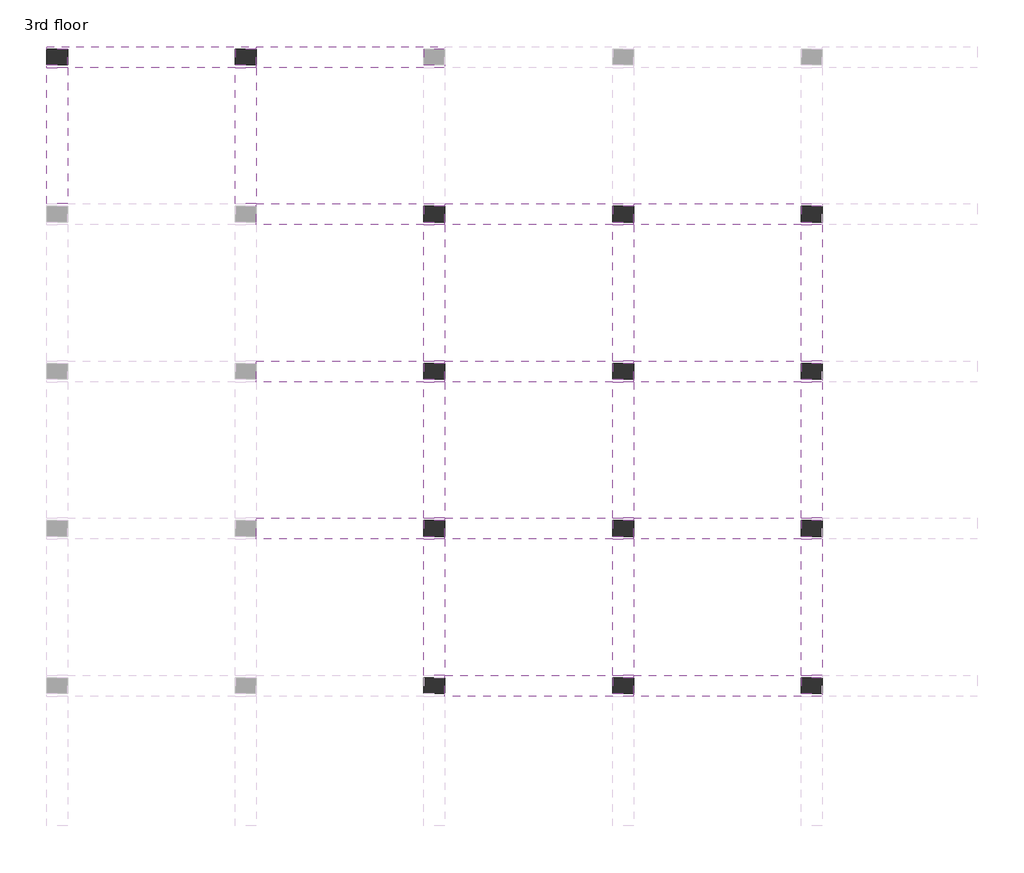
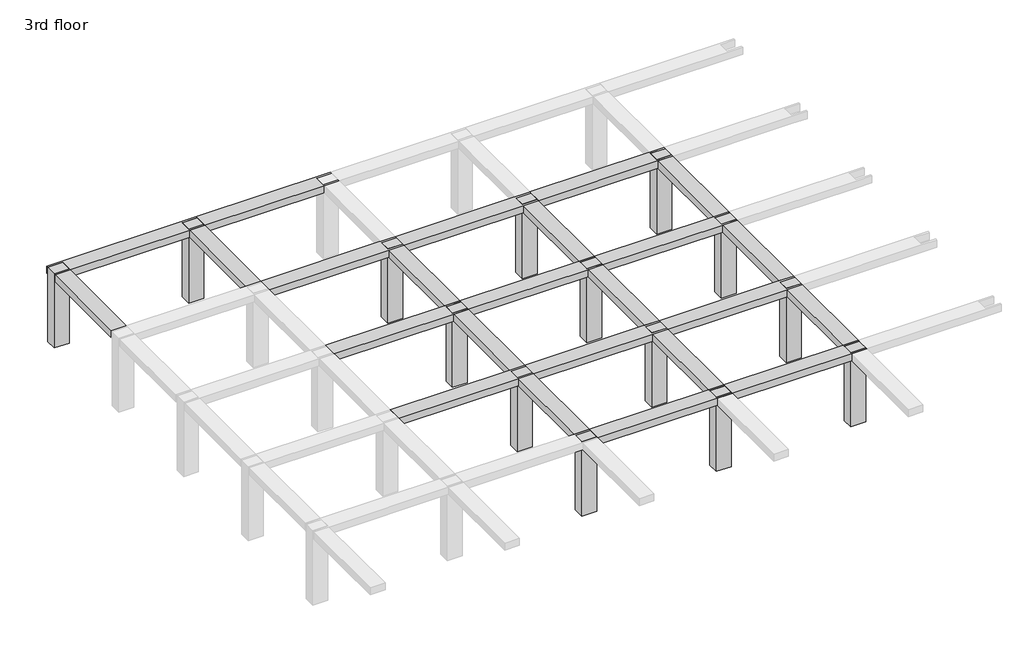
# One storey, part 2 of 3: 24 beams, 14 columns.
"""IFC4 building model written with IfcOpenShell, lengths in millimetres."""

from ifc_helpers import new_model, si_unit, frame, origin, place, context, project, spatial, polyline, outline, extrude, faceted_brep, element, save

model = new_model("IFC4")

# Units and contexts
model_context = context("Model", 3, world=origin())
ifc_project = project(units=[si_unit("LENGTHUNIT", "METRE", prefix="MILLI")], contexts=[model_context])

# Site, building, storey
site = spatial("IfcSite", under=ifc_project)
building = spatial("IfcBuilding", under=site)
storey = spatial("IfcBuildingStorey", under=building, Name="3rd floor", Elevation=9601.2)

# Beams
placement = place(None, origin())
element("IfcBeam", 1, ObjectType="Concrete-Rectangular Beam : 2' x2'", at=placement, inside=storey, context=model_context, shape_type="Brep", body=[
    faceted_brep([(-5646.474232, 1680.7831222, 12801.6), (-6256.074232, 1680.7831222, 12801.6), (-11132.874232, 1680.7831222, 12801.6), (-11132.874232, 1604.5831222, 12801.6), (-11132.874232, 1147.3831222, 12801.6), (-11132.874232, 1071.1831222, 12801.6), (-6256.074232, 1071.1831222, 12801.6), (-5646.474232, 1071.1831222, 12801.6), (-5646.474232, 1147.3831222, 12801.6), (-6256.074232, 1147.3831222, 12801.6), (-6256.074232, 1604.5831222, 12801.6), (-5646.474232, 1604.5831222, 12801.6), (-5646.474232, 1071.1831222, 12496.8), (-11132.874232, 1071.1831222, 12496.8), (-6256.074232, 1071.1831222, 12496.8), (-11132.874232, 1147.3831222, 12496.8), (-11132.874232, 1604.5831222, 12496.8), (-11132.874232, 1680.7831222, 12496.8), (-6256.074232, 1680.7831222, 12496.8), (-5646.474232, 1680.7831222, 12496.8), (-5646.474232, 1604.5831222, 12496.8), (-6256.074232, 1604.5831222, 12496.8), (-6256.074232, 1147.3831222, 12496.8), (-5646.474232, 1147.3831222, 12496.8)], [[[0, 1, 2, 3, 4, 5, 6, 7, 8, 9, 10, 11]], [[12, 7, 6, 5, 13, 14]], [[12, 14, 13, 15, 16, 17, 18, 19, 20, 21, 22, 23]], [[0, 19, 18, 17, 2, 1]], [[7, 12, 23, 8]], [[5, 4, 3, 2, 17, 16, 15, 13]], [[22, 9, 8, 23]], [[9, 22, 21, 10]], [[10, 21, 20, 11]], [[19, 0, 11, 20]]]),
])
element("IfcBeam", 2, ObjectType="Concrete-Rectangular Beam : 2' x2'", at=placement, inside=storey, context=model_context, shape_type="Brep", body=[
    faceted_brep([(-5646.474232, 1680.7831222, 12801.6), (-5646.474232, 1604.5831222, 12801.6), (-5646.474232, 1147.3831222, 12801.6), (-5646.474232, 1071.1831222, 12801.6), (-769.674232, 1071.1831222, 12801.6), (-160.074232, 1071.1831222, 12801.6), (-160.074232, 1147.3831222, 12801.6), (-769.674232, 1147.3831222, 12801.6), (-769.674232, 1604.5831222, 12801.6), (-160.074232, 1604.5831222, 12801.6), (-160.074232, 1680.7831222, 12801.6), (-769.674232, 1680.7831222, 12801.6), (-5646.474232, 1071.1831222, 12496.8), (-769.674232, 1071.1831222, 12496.8), (-160.074232, 1071.1831222, 12496.8), (-5646.474232, 1147.3831222, 12496.8), (-5646.474232, 1604.5831222, 12496.8), (-5646.474232, 1680.7831222, 12496.8), (-769.674232, 1680.7831222, 12496.8), (-160.074232, 1680.7831222, 12496.8), (-160.074232, 1604.5831222, 12496.8), (-769.674232, 1604.5831222, 12496.8), (-769.674232, 1147.3831222, 12496.8), (-160.074232, 1147.3831222, 12496.8)], [[[0, 1, 2, 3, 4, 5, 6, 7, 8, 9, 10, 11]], [[3, 12, 13, 14, 5, 4]], [[12, 15, 16, 17, 18, 19, 20, 21, 22, 23, 14, 13]], [[10, 19, 18, 17, 0, 11]], [[3, 2, 1, 0, 17, 16, 15, 12]], [[5, 14, 23, 6]], [[22, 7, 6, 23]], [[7, 22, 21, 8]], [[8, 21, 20, 9]], [[19, 10, 9, 20]]]),
])
element("IfcBeam", 3, ObjectType="Concrete-Rectangular Beam : 2' x2'", at=placement, inside=storey, context=model_context, shape_type="Brep", body=[
    faceted_brep([(-16619.274232, 6252.7831222, 12801.6), (-16619.274232, 6176.5831222, 12801.6), (-16619.274232, 5719.3831222, 12801.6), (-16619.274232, 5643.1831222, 12801.6), (-11742.474232, 5643.1831222, 12801.6), (-11132.874232, 5643.1831222, 12801.6), (-11132.874232, 5719.3831222, 12801.6), (-11742.474232, 5719.3831222, 12801.6), (-11742.474232, 6176.5831222, 12801.6), (-11132.874232, 6176.5831222, 12801.6), (-11132.874232, 6252.7831222, 12801.6), (-11742.474232, 6252.7831222, 12801.6), (-16619.274232, 5643.1831222, 12496.8), (-11742.474232, 5643.1831222, 12496.8), (-11132.874232, 5643.1831222, 12496.8), (-16619.274232, 5719.3831222, 12496.8), (-16619.274232, 6176.5831222, 12496.8), (-16619.274232, 6252.7831222, 12496.8), (-11742.474232, 6252.7831222, 12496.8), (-11132.874232, 6252.7831222, 12496.8), (-11132.874232, 6176.5831222, 12496.8), (-11742.474232, 6176.5831222, 12496.8), (-11742.474232, 5719.3831222, 12496.8), (-11132.874232, 5719.3831222, 12496.8)], [[[0, 1, 2, 3, 4, 5, 6, 7, 8, 9, 10, 11]], [[3, 12, 13, 14, 5, 4]], [[12, 15, 16, 17, 18, 19, 20, 21, 22, 23, 14, 13]], [[10, 19, 18, 17, 0, 11]], [[3, 2, 1, 0, 17, 16, 15, 12]], [[5, 14, 23, 6]], [[22, 7, 6, 23]], [[7, 22, 21, 8]], [[8, 21, 20, 9]], [[19, 10, 9, 20]]]),
])
element("IfcBeam", 4, ObjectType="Concrete-Rectangular Beam : 2' x2'", at=placement, inside=storey, context=model_context, shape_type="Brep", body=[
    faceted_brep([(-5646.474232, 6252.7831222, 12801.6), (-6256.074232, 6252.7831222, 12801.6), (-11132.874232, 6252.7831222, 12801.6), (-11132.874232, 6176.5831222, 12801.6), (-11132.874232, 5719.3831222, 12801.6), (-11132.874232, 5643.1831222, 12801.6), (-6256.074232, 5643.1831222, 12801.6), (-5646.474232, 5643.1831222, 12801.6), (-5646.474232, 5719.3831222, 12801.6), (-6256.074232, 5719.3831222, 12801.6), (-6256.074232, 6176.5831222, 12801.6), (-5646.474232, 6176.5831222, 12801.6), (-5646.474232, 5643.1831222, 12496.8), (-11132.874232, 5643.1831222, 12496.8), (-6256.074232, 5643.1831222, 12496.8), (-11132.874232, 5719.3831222, 12496.8), (-11132.874232, 6176.5831222, 12496.8), (-11132.874232, 6252.7831222, 12496.8), (-6256.074232, 6252.7831222, 12496.8), (-5646.474232, 6252.7831222, 12496.8), (-5646.474232, 6176.5831222, 12496.8), (-6256.074232, 6176.5831222, 12496.8), (-6256.074232, 5719.3831222, 12496.8), (-5646.474232, 5719.3831222, 12496.8)], [[[0, 1, 2, 3, 4, 5, 6, 7, 8, 9, 10, 11]], [[12, 7, 6, 5, 13, 14]], [[12, 14, 13, 15, 16, 17, 18, 19, 20, 21, 22, 23]], [[0, 19, 18, 17, 2, 1]], [[7, 12, 23, 8]], [[5, 4, 3, 2, 17, 16, 15, 13]], [[22, 9, 8, 23]], [[9, 22, 21, 10]], [[10, 21, 20, 11]], [[19, 0, 11, 20]]]),
])
element("IfcBeam", 5, ObjectType="Concrete-Rectangular Beam : 2' x2'", at=placement, inside=storey, context=model_context, shape_type="Brep", body=[
    faceted_brep([(-5646.474232, 6252.7831222, 12801.6), (-5646.474232, 6176.5831222, 12801.6), (-5646.474232, 5719.3831222, 12801.6), (-5646.474232, 5643.1831222, 12801.6), (-769.674232, 5643.1831222, 12801.6), (-160.074232, 5643.1831222, 12801.6), (-160.074232, 5719.3831222, 12801.6), (-769.674232, 5719.3831222, 12801.6), (-769.674232, 6176.5831222, 12801.6), (-160.074232, 6176.5831222, 12801.6), (-160.074232, 6252.7831222, 12801.6), (-769.674232, 6252.7831222, 12801.6), (-5646.474232, 5643.1831222, 12496.8), (-769.674232, 5643.1831222, 12496.8), (-160.074232, 5643.1831222, 12496.8), (-5646.474232, 5719.3831222, 12496.8), (-5646.474232, 6176.5831222, 12496.8), (-5646.474232, 6252.7831222, 12496.8), (-769.674232, 6252.7831222, 12496.8), (-160.074232, 6252.7831222, 12496.8), (-160.074232, 6176.5831222, 12496.8), (-769.674232, 6176.5831222, 12496.8), (-769.674232, 5719.3831222, 12496.8), (-160.074232, 5719.3831222, 12496.8)], [[[0, 1, 2, 3, 4, 5, 6, 7, 8, 9, 10, 11]], [[3, 12, 13, 14, 5, 4]], [[12, 15, 16, 17, 18, 19, 20, 21, 22, 23, 14, 13]], [[10, 19, 18, 17, 0, 11]], [[3, 2, 1, 0, 17, 16, 15, 12]], [[5, 14, 23, 6]], [[22, 7, 6, 23]], [[7, 22, 21, 8]], [[8, 21, 20, 9]], [[19, 10, 9, 20]]]),
])
element("IfcBeam", 6, ObjectType="Concrete-Rectangular Beam : 2' x2'", at=placement, inside=storey, context=model_context, shape_type="Brep", body=[
    faceted_brep([(-16619.274232, 10824.7831222, 12801.6), (-16619.274232, 10748.5831222, 12801.6), (-16619.274232, 10291.3831222, 12801.6), (-16619.274232, 10215.1831222, 12801.6), (-11742.474232, 10215.1831222, 12801.6), (-11132.874232, 10215.1831222, 12801.6), (-11132.874232, 10291.3831222, 12801.6), (-11742.474232, 10291.3831222, 12801.6), (-11742.474232, 10748.5831222, 12801.6), (-11132.874232, 10748.5831222, 12801.6), (-11132.874232, 10824.7831222, 12801.6), (-11742.474232, 10824.7831222, 12801.6), (-16619.274232, 10215.1831222, 12496.8), (-11742.474232, 10215.1831222, 12496.8), (-11132.874232, 10215.1831222, 12496.8), (-16619.274232, 10291.3831222, 12496.8), (-16619.274232, 10748.5831222, 12496.8), (-16619.274232, 10824.7831222, 12496.8), (-11742.474232, 10824.7831222, 12496.8), (-11132.874232, 10824.7831222, 12496.8), (-11132.874232, 10748.5831222, 12496.8), (-11742.474232, 10748.5831222, 12496.8), (-11742.474232, 10291.3831222, 12496.8), (-11132.874232, 10291.3831222, 12496.8)], [[[0, 1, 2, 3, 4, 5, 6, 7, 8, 9, 10, 11]], [[3, 12, 13, 14, 5, 4]], [[12, 15, 16, 17, 18, 19, 20, 21, 22, 23, 14, 13]], [[10, 19, 18, 17, 0, 11]], [[3, 2, 1, 0, 17, 16, 15, 12]], [[5, 14, 23, 6]], [[22, 7, 6, 23]], [[7, 22, 21, 8]], [[8, 21, 20, 9]], [[19, 10, 9, 20]]]),
])
element("IfcBeam", 7, ObjectType="Concrete-Rectangular Beam : 2' x2'", at=placement, inside=storey, context=model_context, shape_type="Brep", body=[
    faceted_brep([(-11132.874232, 10824.7831222, 12801.6), (-11132.874232, 10748.5831222, 12801.6), (-11132.874232, 10291.3831222, 12801.6), (-11132.874232, 10215.1831222, 12801.6), (-6256.074232, 10215.1831222, 12801.6), (-5646.474232, 10215.1831222, 12801.6), (-5646.474232, 10291.3831222, 12801.6), (-6256.074232, 10291.3831222, 12801.6), (-6256.074232, 10748.5831222, 12801.6), (-5646.474232, 10748.5831222, 12801.6), (-5646.474232, 10824.7831222, 12801.6), (-6256.074232, 10824.7831222, 12801.6), (-11132.874232, 10215.1831222, 12496.8), (-6256.074232, 10215.1831222, 12496.8), (-5646.474232, 10215.1831222, 12496.8), (-11132.874232, 10291.3831222, 12496.8), (-11132.874232, 10748.5831222, 12496.8), (-11132.874232, 10824.7831222, 12496.8), (-6256.074232, 10824.7831222, 12496.8), (-5646.474232, 10824.7831222, 12496.8), (-5646.474232, 10748.5831222, 12496.8), (-6256.074232, 10748.5831222, 12496.8), (-6256.074232, 10291.3831222, 12496.8), (-5646.474232, 10291.3831222, 12496.8)], [[[0, 1, 2, 3, 4, 5, 6, 7, 8, 9, 10, 11]], [[3, 12, 13, 14, 5, 4]], [[12, 15, 16, 17, 18, 19, 20, 21, 22, 23, 14, 13]], [[10, 19, 18, 17, 0, 11]], [[3, 2, 1, 0, 17, 16, 15, 12]], [[5, 14, 23, 6]], [[22, 7, 6, 23]], [[7, 22, 21, 8]], [[8, 21, 20, 9]], [[19, 10, 9, 20]]]),
])
element("IfcBeam", 8, ObjectType="Concrete-Rectangular Beam : 2' x2'", at=placement, inside=storey, context=model_context, shape_type="Brep", body=[
    faceted_brep([(-5646.474232, 10824.7831222, 12801.6), (-5646.474232, 10748.5831222, 12801.6), (-5646.474232, 10291.3831222, 12801.6), (-5646.474232, 10215.1831222, 12801.6), (-769.674232, 10215.1831222, 12801.6), (-160.074232, 10215.1831222, 12801.6), (-160.074232, 10291.3831222, 12801.6), (-769.674232, 10291.3831222, 12801.6), (-769.674232, 10748.5831222, 12801.6), (-160.074232, 10748.5831222, 12801.6), (-160.074232, 10824.7831222, 12801.6), (-769.674232, 10824.7831222, 12801.6), (-5646.474232, 10215.1831222, 12496.8), (-769.674232, 10215.1831222, 12496.8), (-160.074232, 10215.1831222, 12496.8), (-5646.474232, 10291.3831222, 12496.8), (-5646.474232, 10748.5831222, 12496.8), (-5646.474232, 10824.7831222, 12496.8), (-769.674232, 10824.7831222, 12496.8), (-160.074232, 10824.7831222, 12496.8), (-160.074232, 10748.5831222, 12496.8), (-769.674232, 10748.5831222, 12496.8), (-769.674232, 10291.3831222, 12496.8), (-160.074232, 10291.3831222, 12496.8)], [[[0, 1, 2, 3, 4, 5, 6, 7, 8, 9, 10, 11]], [[3, 12, 13, 14, 5, 4]], [[12, 15, 16, 17, 18, 19, 20, 21, 22, 23, 14, 13]], [[10, 19, 18, 17, 0, 11]], [[3, 2, 1, 0, 17, 16, 15, 12]], [[5, 14, 23, 6]], [[22, 7, 6, 23]], [[7, 22, 21, 8]], [[8, 21, 20, 9]], [[19, 10, 9, 20]]]),
])
element("IfcBeam", 9, ObjectType="Concrete-Rectangular Beam : 2' x2'", at=placement, inside=storey, context=model_context, shape_type="Brep", body=[
    faceted_brep([(-16619.274232, 15396.7831222, 12801.6), (-16619.274232, 15320.5831222, 12801.6), (-16619.274232, 14863.3831222, 12801.6), (-16619.274232, 14787.1831222, 12801.6), (-11742.474232, 14787.1831222, 12801.6), (-11132.874232, 14787.1831222, 12801.6), (-11132.874232, 14863.3831222, 12801.6), (-11742.474232, 14863.3831222, 12801.6), (-11742.474232, 15320.5831222, 12801.6), (-11132.874232, 15320.5831222, 12801.6), (-11132.874232, 15396.7831222, 12801.6), (-11742.474232, 15396.7831222, 12801.6), (-16619.274232, 14787.1831222, 12496.8), (-11742.474232, 14787.1831222, 12496.8), (-11132.874232, 14787.1831222, 12496.8), (-16619.274232, 14863.3831222, 12496.8), (-16619.274232, 15320.5831222, 12496.8), (-16619.274232, 15396.7831222, 12496.8), (-11742.474232, 15396.7831222, 12496.8), (-11132.874232, 15396.7831222, 12496.8), (-11132.874232, 15320.5831222, 12496.8), (-11742.474232, 15320.5831222, 12496.8), (-11742.474232, 14863.3831222, 12496.8), (-11132.874232, 14863.3831222, 12496.8)], [[[0, 1, 2, 3, 4, 5, 6, 7, 8, 9, 10, 11]], [[3, 12, 13, 14, 5, 4]], [[12, 15, 16, 17, 18, 19, 20, 21, 22, 23, 14, 13]], [[10, 19, 18, 17, 0, 11]], [[3, 2, 1, 0, 17, 16, 15, 12]], [[5, 14, 23, 6]], [[22, 7, 6, 23]], [[7, 22, 21, 8]], [[8, 21, 20, 9]], [[19, 10, 9, 20]]]),
])
element("IfcBeam", 10, ObjectType="Concrete-Rectangular Beam : 2' x2'", at=placement, inside=storey, context=model_context, shape_type="Brep", body=[
    faceted_brep([(-11132.874232, 15396.7831222, 12801.6), (-11132.874232, 15320.5831222, 12801.6), (-11132.874232, 14863.3831222, 12801.6), (-11132.874232, 14787.1831222, 12801.6), (-6256.074232, 14787.1831222, 12801.6), (-5646.474232, 14787.1831222, 12801.6), (-5646.474232, 14863.3831222, 12801.6), (-6256.074232, 14863.3831222, 12801.6), (-6256.074232, 15320.5831222, 12801.6), (-5646.474232, 15320.5831222, 12801.6), (-5646.474232, 15396.7831222, 12801.6), (-6256.074232, 15396.7831222, 12801.6), (-11132.874232, 14787.1831222, 12496.8), (-6256.074232, 14787.1831222, 12496.8), (-5646.474232, 14787.1831222, 12496.8), (-11132.874232, 14863.3831222, 12496.8), (-11132.874232, 15320.5831222, 12496.8), (-11132.874232, 15396.7831222, 12496.8), (-6256.074232, 15396.7831222, 12496.8), (-5646.474232, 15396.7831222, 12496.8), (-5646.474232, 15320.5831222, 12496.8), (-6256.074232, 15320.5831222, 12496.8), (-6256.074232, 14863.3831222, 12496.8), (-5646.474232, 14863.3831222, 12496.8)], [[[0, 1, 2, 3, 4, 5, 6, 7, 8, 9, 10, 11]], [[3, 12, 13, 14, 5, 4]], [[12, 15, 16, 17, 18, 19, 20, 21, 22, 23, 14, 13]], [[10, 19, 18, 17, 0, 11]], [[3, 2, 1, 0, 17, 16, 15, 12]], [[5, 14, 23, 6]], [[22, 7, 6, 23]], [[7, 22, 21, 8]], [[8, 21, 20, 9]], [[19, 10, 9, 20]]]),
])
element("IfcBeam", 11, ObjectType="Concrete-Rectangular Beam : 2' x2'", at=placement, inside=storey, context=model_context, shape_type="Brep", body=[
    faceted_brep([(-5646.474232, 15396.7831222, 12801.6), (-5646.474232, 15320.5831222, 12801.6), (-5646.474232, 14863.3831222, 12801.6), (-5646.474232, 14787.1831222, 12801.6), (-769.674232, 14787.1831222, 12801.6), (-160.074232, 14787.1831222, 12801.6), (-160.074232, 14863.3831222, 12801.6), (-769.674232, 14863.3831222, 12801.6), (-769.674232, 15320.5831222, 12801.6), (-160.074232, 15320.5831222, 12801.6), (-160.074232, 15396.7831222, 12801.6), (-769.674232, 15396.7831222, 12801.6), (-5646.474232, 14787.1831222, 12496.8), (-769.674232, 14787.1831222, 12496.8), (-160.074232, 14787.1831222, 12496.8), (-5646.474232, 14863.3831222, 12496.8), (-5646.474232, 15320.5831222, 12496.8), (-5646.474232, 15396.7831222, 12496.8), (-769.674232, 15396.7831222, 12496.8), (-160.074232, 15396.7831222, 12496.8), (-160.074232, 15320.5831222, 12496.8), (-769.674232, 15320.5831222, 12496.8), (-769.674232, 14863.3831222, 12496.8), (-160.074232, 14863.3831222, 12496.8)], [[[0, 1, 2, 3, 4, 5, 6, 7, 8, 9, 10, 11]], [[3, 12, 13, 14, 5, 4]], [[12, 15, 16, 17, 18, 19, 20, 21, 22, 23, 14, 13]], [[10, 19, 18, 17, 0, 11]], [[3, 2, 1, 0, 17, 16, 15, 12]], [[5, 14, 23, 6]], [[22, 7, 6, 23]], [[7, 22, 21, 8]], [[8, 21, 20, 9]], [[19, 10, 9, 20]]]),
])
element("IfcBeam", 12, ObjectType="Concrete-Rectangular Beam : 2' x2'", at=placement, inside=storey, context=model_context, shape_type="Brep", body=[
    faceted_brep([(-16619.274232, 19968.7831222, 12801.6), (-22715.274232, 19968.7831222, 12801.6), (-22715.274232, 19892.5831222, 12801.6), (-22105.674232, 19892.5831222, 12801.6), (-22105.674232, 19435.3831222, 12801.6), (-22715.274232, 19435.3831222, 12801.6), (-22715.274232, 19359.1831222, 12801.6), (-22105.674232, 19359.1831222, 12801.6), (-17228.874232, 19359.1831222, 12801.6), (-16619.274232, 19359.1831222, 12801.6), (-16619.274232, 19435.3831222, 12801.6), (-17228.874232, 19435.3831222, 12801.6), (-17228.874232, 19892.5831222, 12801.6), (-16619.274232, 19892.5831222, 12801.6), (-22715.274232, 19359.1831222, 12496.8), (-22105.674232, 19359.1831222, 12496.8), (-17228.874232, 19359.1831222, 12496.8), (-16619.274232, 19359.1831222, 12496.8), (-22715.274232, 19435.3831222, 12496.8), (-22105.674232, 19435.3831222, 12496.8), (-22105.674232, 19892.5831222, 12496.8), (-22715.274232, 19892.5831222, 12496.8), (-22715.274232, 19968.7831222, 12496.8), (-16619.274232, 19968.7831222, 12496.8), (-16619.274232, 19892.5831222, 12496.8), (-17228.874232, 19892.5831222, 12496.8), (-17228.874232, 19435.3831222, 12496.8), (-16619.274232, 19435.3831222, 12496.8)], [[[0, 1, 2, 3, 4, 5, 6, 7, 8, 9, 10, 11, 12, 13]], [[6, 14, 15, 16, 17, 9, 8, 7]], [[17, 16, 15, 14, 18, 19, 20, 21, 22, 23, 24, 25, 26, 27]], [[22, 1, 0, 23]], [[14, 6, 5, 18]], [[9, 17, 27, 10]], [[19, 4, 3, 20]], [[4, 19, 18, 5]], [[20, 3, 2, 21]], [[1, 22, 21, 2]], [[26, 11, 10, 27]], [[11, 26, 25, 12]], [[12, 25, 24, 13]], [[23, 0, 13, 24]]]),
])
element("IfcBeam", 13, ObjectType="Concrete-Rectangular Beam : 2' x2'", at=placement, inside=storey, context=model_context, shape_type="Brep", body=[
    faceted_brep([(-11132.874232, 19968.7831222, 12801.6), (-16619.274232, 19968.7831222, 12801.6), (-16619.274232, 19892.5831222, 12801.6), (-16619.274232, 19435.3831222, 12801.6), (-16619.274232, 19359.1831222, 12801.6), (-11742.474232, 19359.1831222, 12801.6), (-11132.874232, 19359.1831222, 12801.6), (-11132.874232, 19435.3831222, 12801.6), (-11742.474232, 19435.3831222, 12801.6), (-11742.474232, 19892.5831222, 12801.6), (-11132.874232, 19892.5831222, 12801.6), (-11132.874232, 19359.1831222, 12496.8), (-16619.274232, 19359.1831222, 12496.8), (-11742.474232, 19359.1831222, 12496.8), (-16619.274232, 19435.3831222, 12496.8), (-16619.274232, 19892.5831222, 12496.8), (-16619.274232, 19968.7831222, 12496.8), (-11132.874232, 19968.7831222, 12496.8), (-11132.874232, 19892.5831222, 12496.8), (-11742.474232, 19892.5831222, 12496.8), (-11742.474232, 19435.3831222, 12496.8), (-11132.874232, 19435.3831222, 12496.8)], [[[0, 1, 2, 3, 4, 5, 6, 7, 8, 9, 10]], [[11, 6, 5, 4, 12, 13]], [[11, 13, 12, 14, 15, 16, 17, 18, 19, 20, 21]], [[0, 17, 16, 1]], [[6, 11, 21, 7]], [[4, 3, 2, 1, 16, 15, 14, 12]], [[20, 8, 7, 21]], [[8, 20, 19, 9]], [[9, 19, 18, 10]], [[17, 0, 10, 18]]]),
])
element("IfcBeam", 14, ObjectType="Concrete-Rectangular Beam : 2' x2'", at=placement, inside=storey, context=model_context, shape_type="SweptSolid", body=[
    extrude(outline(polyline([(-22105.674232, 15396.7831222), (-22715.274232, 15396.7831222), (-22715.274232, 19359.1831222), (-22105.674232, 19359.1831222), (-22105.674232, 15396.7831222)])), frame((0.0, 0.0, 12496.8), z_axis=(0.0, 0.0, 1.0), x_axis=(1.0, 0.0, 0.0)), (0.0, 0.0, 1.0), 304.8),
])
element("IfcBeam", 15, ObjectType="Concrete-Rectangular Beam : 2' x2'", at=placement, inside=storey, context=model_context, shape_type="SweptSolid", body=[
    extrude(outline(polyline([(-16619.274232, 15396.7831222), (-17228.874232, 15396.7831222), (-17228.874232, 19359.1831222), (-16619.274232, 19359.1831222), (-16619.274232, 15396.7831222)])), frame((0.0, 0.0, 12496.8), z_axis=(0.0, 0.0, 1.0), x_axis=(1.0, 0.0, 0.0)), (0.0, 0.0, 1.0), 304.8),
])
element("IfcBeam", 16, ObjectType="Concrete-Rectangular Beam : 2' x2'", at=placement, inside=storey, context=model_context, shape_type="SweptSolid", body=[
    extrude(outline(polyline([(-11132.874232, 1680.7831222), (-11742.474232, 1680.7831222), (-11742.474232, 5643.1831222), (-11132.874232, 5643.1831222), (-11132.874232, 1680.7831222)])), frame((0.0, 0.0, 12496.8), z_axis=(0.0, 0.0, 1.0), x_axis=(1.0, 0.0, 0.0)), (0.0, 0.0, 1.0), 304.8),
])
element("IfcBeam", 17, ObjectType="Concrete-Rectangular Beam : 2' x2'", at=placement, inside=storey, context=model_context, shape_type="SweptSolid", body=[
    extrude(outline(polyline([(-11132.874232, 6252.7831222), (-11742.474232, 6252.7831222), (-11742.474232, 10215.1831222), (-11132.874232, 10215.1831222), (-11132.874232, 6252.7831222)])), frame((0.0, 0.0, 12496.8), z_axis=(0.0, 0.0, 1.0), x_axis=(1.0, 0.0, 0.0)), (0.0, 0.0, 1.0), 304.8),
])
element("IfcBeam", 18, ObjectType="Concrete-Rectangular Beam : 2' x2'", at=placement, inside=storey, context=model_context, shape_type="SweptSolid", body=[
    extrude(outline(polyline([(-11132.874232, 10824.7831222), (-11742.474232, 10824.7831222), (-11742.474232, 14787.1831222), (-11132.874232, 14787.1831222), (-11132.874232, 10824.7831222)])), frame((0.0, 0.0, 12496.8), z_axis=(0.0, 0.0, 1.0), x_axis=(1.0, 0.0, 0.0)), (0.0, 0.0, 1.0), 304.8),
])
element("IfcBeam", 19, ObjectType="Concrete-Rectangular Beam : 2' x2'", at=placement, inside=storey, context=model_context, shape_type="SweptSolid", body=[
    extrude(outline(polyline([(-5646.474232, 1680.7831222), (-6256.074232, 1680.7831222), (-6256.074232, 5643.1831222), (-5646.474232, 5643.1831222), (-5646.474232, 1680.7831222)])), frame((0.0, 0.0, 12496.8), z_axis=(0.0, 0.0, 1.0), x_axis=(1.0, 0.0, 0.0)), (0.0, 0.0, 1.0), 304.8),
])
element("IfcBeam", 20, ObjectType="Concrete-Rectangular Beam : 2' x2'", at=placement, inside=storey, context=model_context, shape_type="SweptSolid", body=[
    extrude(outline(polyline([(-5646.474232, 6252.7831222), (-6256.074232, 6252.7831222), (-6256.074232, 10215.1831222), (-5646.474232, 10215.1831222), (-5646.474232, 6252.7831222)])), frame((0.0, 0.0, 12496.8), z_axis=(0.0, 0.0, 1.0), x_axis=(1.0, 0.0, 0.0)), (0.0, 0.0, 1.0), 304.8),
])
element("IfcBeam", 21, ObjectType="Concrete-Rectangular Beam : 2' x2'", at=placement, inside=storey, context=model_context, shape_type="SweptSolid", body=[
    extrude(outline(polyline([(-5646.474232, 10824.7831222), (-6256.074232, 10824.7831222), (-6256.074232, 14787.1831222), (-5646.474232, 14787.1831222), (-5646.474232, 10824.7831222)])), frame((0.0, 0.0, 12496.8), z_axis=(0.0, 0.0, 1.0), x_axis=(1.0, 0.0, 0.0)), (0.0, 0.0, 1.0), 304.8),
])
element("IfcBeam", 22, ObjectType="Concrete-Rectangular Beam : 2' x2'", at=placement, inside=storey, context=model_context, shape_type="SweptSolid", body=[
    extrude(outline(polyline([(-769.674232, 5643.1831222), (-160.074232, 5643.1831222), (-160.074232, 1680.7831222), (-769.674232, 1680.7831222), (-769.674232, 5643.1831222)])), frame((0.0, 0.0, 12496.8), z_axis=(0.0, 0.0, 1.0), x_axis=(1.0, 0.0, 0.0)), (0.0, 0.0, 1.0), 304.8),
])
element("IfcBeam", 23, ObjectType="Concrete-Rectangular Beam : 2' x2'", at=placement, inside=storey, context=model_context, shape_type="SweptSolid", body=[
    extrude(outline(polyline([(-160.074232, 6252.7831222), (-769.674232, 6252.7831222), (-769.674232, 10215.1831222), (-160.074232, 10215.1831222), (-160.074232, 6252.7831222)])), frame((0.0, 0.0, 12496.8), z_axis=(0.0, 0.0, 1.0), x_axis=(1.0, 0.0, 0.0)), (0.0, 0.0, 1.0), 304.8),
])
element("IfcBeam", 24, ObjectType="Concrete-Rectangular Beam : 2' x2'", at=placement, inside=storey, context=model_context, shape_type="SweptSolid", body=[
    extrude(outline(polyline([(-769.674232, 14787.1831222), (-160.074232, 14787.1831222), (-160.074232, 10824.7831222), (-769.674232, 10824.7831222), (-769.674232, 14787.1831222)])), frame((0.0, 0.0, 12496.8), z_axis=(0.0, 0.0, 1.0), x_axis=(1.0, 0.0, 0.0)), (0.0, 0.0, 1.0), 304.8),
])

# Columns
element("IfcColumn", 25, ObjectType="Concrete-Rectangular-Column : 12 x 18", at=placement, inside=storey, context=model_context, shape_type="SweptSolid", body=[
    extrude(outline(polyline([(-11132.874232, 1604.5831222), (-11132.874232, 1147.3831222), (-11742.474232, 1147.3831222), (-11742.474232, 1604.5831222), (-11132.874232, 1604.5831222)])), frame((0.0, 0.0, 9601.2), z_axis=(0.0, 0.0, 1.0), x_axis=(1.0, 0.0, 0.0)), (0.0, 0.0, 1.0), 3200.4),
])
element("IfcColumn", 26, ObjectType="Concrete-Rectangular-Column : 12 x 18", at=placement, inside=storey, context=model_context, shape_type="SweptSolid", body=[
    extrude(outline(polyline([(-5646.474232, 1604.5831222), (-5646.474232, 1147.3831222), (-6256.074232, 1147.3831222), (-6256.074232, 1604.5831222), (-5646.474232, 1604.5831222)])), frame((0.0, 0.0, 9601.2), z_axis=(0.0, 0.0, 1.0), x_axis=(1.0, 0.0, 0.0)), (0.0, 0.0, 1.0), 3200.4),
])
element("IfcColumn", 27, ObjectType="Concrete-Rectangular-Column : 12 x 18", at=placement, inside=storey, context=model_context, shape_type="SweptSolid", body=[
    extrude(outline(polyline([(-160.074232, 1604.5831222), (-160.074232, 1147.3831222), (-769.674232, 1147.3831222), (-769.674232, 1604.5831222), (-160.074232, 1604.5831222)])), frame((0.0, 0.0, 9601.2), z_axis=(0.0, 0.0, 1.0), x_axis=(1.0, 0.0, 0.0)), (0.0, 0.0, 1.0), 3200.4),
])
element("IfcColumn", 28, ObjectType="Concrete-Rectangular-Column : 12 x 18", at=placement, inside=storey, context=model_context, shape_type="SweptSolid", body=[
    extrude(outline(polyline([(-11132.874232, 6176.5831222), (-11132.874232, 5719.3831222), (-11742.474232, 5719.3831222), (-11742.474232, 6176.5831222), (-11132.874232, 6176.5831222)])), frame((0.0, 0.0, 9601.2), z_axis=(0.0, 0.0, 1.0), x_axis=(1.0, 0.0, 0.0)), (0.0, 0.0, 1.0), 3200.4),
])
element("IfcColumn", 29, ObjectType="Concrete-Rectangular-Column : 12 x 18", at=placement, inside=storey, context=model_context, shape_type="SweptSolid", body=[
    extrude(outline(polyline([(-5646.474232, 6176.5831222), (-5646.474232, 5719.3831222), (-6256.074232, 5719.3831222), (-6256.074232, 6176.5831222), (-5646.474232, 6176.5831222)])), frame((0.0, 0.0, 9601.2), z_axis=(0.0, 0.0, 1.0), x_axis=(1.0, 0.0, 0.0)), (0.0, 0.0, 1.0), 3200.4),
])
element("IfcColumn", 30, ObjectType="Concrete-Rectangular-Column : 12 x 18", at=placement, inside=storey, context=model_context, shape_type="SweptSolid", body=[
    extrude(outline(polyline([(-160.074232, 6176.5831222), (-160.074232, 5719.3831222), (-769.674232, 5719.3831222), (-769.674232, 6176.5831222), (-160.074232, 6176.5831222)])), frame((0.0, 0.0, 9601.2), z_axis=(0.0, 0.0, 1.0), x_axis=(1.0, 0.0, 0.0)), (0.0, 0.0, 1.0), 3200.4),
])
element("IfcColumn", 31, ObjectType="Concrete-Rectangular-Column : 12 x 18", at=placement, inside=storey, context=model_context, shape_type="SweptSolid", body=[
    extrude(outline(polyline([(-11132.874232, 10748.5831222), (-11132.874232, 10291.3831222), (-11742.474232, 10291.3831222), (-11742.474232, 10748.5831222), (-11132.874232, 10748.5831222)])), frame((0.0, 0.0, 9601.2), z_axis=(0.0, 0.0, 1.0), x_axis=(1.0, 0.0, 0.0)), (0.0, 0.0, 1.0), 3200.4),
])
element("IfcColumn", 32, ObjectType="Concrete-Rectangular-Column : 12 x 18", at=placement, inside=storey, context=model_context, shape_type="SweptSolid", body=[
    extrude(outline(polyline([(-5646.474232, 10748.5831222), (-5646.474232, 10291.3831222), (-6256.074232, 10291.3831222), (-6256.074232, 10748.5831222), (-5646.474232, 10748.5831222)])), frame((0.0, 0.0, 9601.2), z_axis=(0.0, 0.0, 1.0), x_axis=(1.0, 0.0, 0.0)), (0.0, 0.0, 1.0), 3200.4),
])
element("IfcColumn", 33, ObjectType="Concrete-Rectangular-Column : 12 x 18", at=placement, inside=storey, context=model_context, shape_type="SweptSolid", body=[
    extrude(outline(polyline([(-160.074232, 10748.5831222), (-160.074232, 10291.3831222), (-769.674232, 10291.3831222), (-769.674232, 10748.5831222), (-160.074232, 10748.5831222)])), frame((0.0, 0.0, 9601.2), z_axis=(0.0, 0.0, 1.0), x_axis=(1.0, 0.0, 0.0)), (0.0, 0.0, 1.0), 3200.4),
])
element("IfcColumn", 34, ObjectType="Concrete-Rectangular-Column : 12 x 18", at=placement, inside=storey, context=model_context, shape_type="SweptSolid", body=[
    extrude(outline(polyline([(-11132.874232, 15320.5831222), (-11132.874232, 14863.3831222), (-11742.474232, 14863.3831222), (-11742.474232, 15320.5831222), (-11132.874232, 15320.5831222)])), frame((0.0, 0.0, 9601.2), z_axis=(0.0, 0.0, 1.0), x_axis=(1.0, 0.0, 0.0)), (0.0, 0.0, 1.0), 3200.4),
])
element("IfcColumn", 35, ObjectType="Concrete-Rectangular-Column : 12 x 18", at=placement, inside=storey, context=model_context, shape_type="SweptSolid", body=[
    extrude(outline(polyline([(-5646.474232, 15320.5831222), (-5646.474232, 14863.3831222), (-6256.074232, 14863.3831222), (-6256.074232, 15320.5831222), (-5646.474232, 15320.5831222)])), frame((0.0, 0.0, 9601.2), z_axis=(0.0, 0.0, 1.0), x_axis=(1.0, 0.0, 0.0)), (0.0, 0.0, 1.0), 3200.4),
])
element("IfcColumn", 36, ObjectType="Concrete-Rectangular-Column : 12 x 18", at=placement, inside=storey, context=model_context, shape_type="SweptSolid", body=[
    extrude(outline(polyline([(-160.074232, 15320.5831222), (-160.074232, 14863.3831222), (-769.674232, 14863.3831222), (-769.674232, 15320.5831222), (-160.074232, 15320.5831222)])), frame((0.0, 0.0, 9601.2), z_axis=(0.0, 0.0, 1.0), x_axis=(1.0, 0.0, 0.0)), (0.0, 0.0, 1.0), 3200.4),
])
element("IfcColumn", 37, ObjectType="Concrete-Rectangular-Column : 12 x 18", at=placement, inside=storey, context=model_context, shape_type="SweptSolid", body=[
    extrude(outline(polyline([(-22105.674232, 19892.5831222), (-22105.674232, 19435.3831222), (-22715.274232, 19435.3831222), (-22715.274232, 19892.5831222), (-22105.674232, 19892.5831222)])), frame((0.0, 0.0, 9601.2), z_axis=(0.0, 0.0, 1.0), x_axis=(1.0, 0.0, 0.0)), (0.0, 0.0, 1.0), 3200.4),
])
element("IfcColumn", 38, ObjectType="Concrete-Rectangular-Column : 12 x 18", at=placement, inside=storey, context=model_context, shape_type="SweptSolid", body=[
    extrude(outline(polyline([(-16619.274232, 19892.5831222), (-16619.274232, 19435.3831222), (-17228.874232, 19435.3831222), (-17228.874232, 19892.5831222), (-16619.274232, 19892.5831222)])), frame((0.0, 0.0, 9601.2), z_axis=(0.0, 0.0, 1.0), x_axis=(1.0, 0.0, 0.0)), (0.0, 0.0, 1.0), 3200.4),
])

save(model, "model.ifc")

# Revit data of these elements
# Type "Concrete-Rectangular Beam : 2' x2'"
#   Assembly Code = "B10"
#   Length [instance default] = 5' - 0"
#   b = 2' - 0"
#   h = 1' - 0"
#   Structural Material [instance default] = Concrete, Cast-in-Place gray
# Type "Concrete-Rectangular-Column : 12 x 18"
#   Assembly Code = "B10"
#   b = 2' - 0"
#   h = 1' - 6"
#   Structural Material [instance default] = Concrete, Cast-in-Place gray
# Elements 1, 2, 3, 4, 5, 6, 7, 8, 9, 10, 11, 12, 13, 14, 15, 16, 17, 18, 19, 20, 21, 22, 23, 24 (IfcBeam, "Concrete-Rectangular Beam : 2' x2'")
#   Structural Material = Concrete, Precast (2)
#   Phase Created = New Construction
#   Materials on its faces: "Concrete, Precast (2)"
# Elements 25, 26, 27, 28, 29, 30, 31, 32, 33, 34, 35, 36, 37, 38 (IfcColumn, "Concrete-Rectangular-Column : 12 x 18")
#   Phase Created = New Construction
#   Materials on its faces: "Concrete, Cast-in-Place gray"
# Materials
#   "Concrete, Cast-in-Place gray": class "Concrete", colour RGB 192 192 192, transparency 0, Description = "Cast-in-place concrete", Cost = 0
#   "Concrete, Precast (2)": class "Concrete", colour RGB 198 187 187, transparency 0, Description = "Precast concrete", Cost = 0
